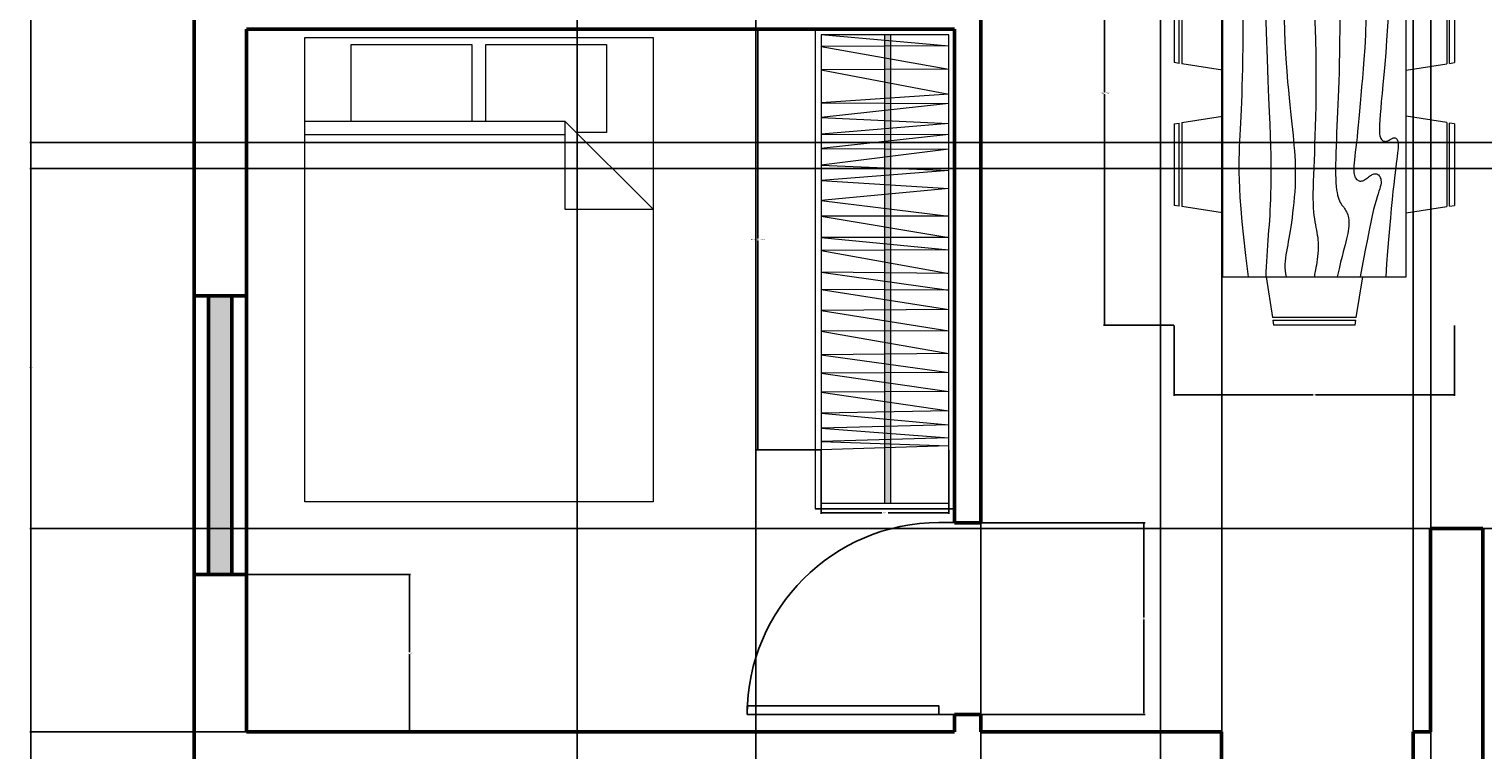
# Model space of a CAD drawing. Units: inches. Extents: x 1974 to 2406, y 1583 to 2170.
# Tile 3 of 6: x 1974 to 2224, y 1806 to 1930. Entities that reach past the tile are written whole.
import ezdxf

# ---------------------------------------------------------------- set-up
doc = ezdxf.new("R2010")
doc.units = ezdxf.units.IN
for name, color, linetype, lineweight in [('A-ANNO-DIMS', 2, 'Continuous', 18), ('A-FURN', 3, 'Continuous', 18), ('A-GLAZ', 4, 'Continuous', 25), ('door', 60, 'Continuous', 25), ('wall', 240, 'Continuous', 50)]:
    doc.layers.add(name, color=color, linetype=linetype, lineweight=lineweight)
doc.layers.add('A-FLOR-CASE', color=40, linetype='Continuous', lineweight=18, true_color=0xf8d731)
doc.layers.add('A-FLOR-CASE-PATT', color=40, linetype='Continuous', lineweight=13, true_color=0xf8d731)
doc.styles.get("Standard").update_dxf_attribs({"font": 'arial.ttf'})
doc.dimstyles.get("Standard").update_dxf_attribs({"dimtxt": 0.18, "dimasz": 0.18, "dimexe": 0.18, "dimexo": 0.0625, "dimgap": 0.09, "dimtad": 0, "dimtih": 1, "dimtoh": 1, "dimdec": 4, "dimzin": 0, "dimdsep": 46, "dimtxsty": 'Standard', "dimcen": 0.09, "dimadec": 0, "dimazin": 0, "dimtfac": 1, "dimtdec": 4, "dimtofl": 0, "dimtmove": 0, "dimatfit": 3, "dimfxl": 1, "dimtolj": 1, "dimtzin": 0, "dimarcsym": 0})

# ---------------------------------------------------------------- blocks, each defined once
blk = doc.blocks.new('*U2')
for p, q in [((0, 0), (0, -6)), ((40, 0), (40, -6))]:
    blk.add_line(p, q)
blk.add_lwpolyline([(0, 0), (0, 40), (1.75, 40), (1.75, 0)], close=True)
blk.add_arc((0, 0), 40, 0, 90)
blk = doc.blocks.new('b')
at = {"layer": 'wall'}
h = blk.add_hatch(color=256, dxfattribs=at)
h.dxf.hatch_style = 1
h.paths.add_polyline_path([(6.5, 0), (2.5, 0), (2.5, -48), (6.5, -48)])
for p, q in [((2.5, 0), (2.5, -48)), ((6.5, 0), (6.5, -48))]:
    blk.add_line(p, q, dxfattribs=at)
blk.add_lwpolyline([(0, -48), (9, -48), (9, 0), (0, 0)], close=True, dxfattribs=at)
blk = doc.blocks.new('Dining Set - 36 x 72 in.')
for p, q in [((-22.2343, 26.00059), (-23.4847, 17.99762)), ((-22.2304, 26), (-5.7608, 26)), ((-22, 27.5), (-22.1562, 26.50042)), ((-5.8416, 26.5), (-22.1534, 26.5)), ((-22, 27.5), (-6, 27.5)), ((-5.8437, 26.49966), (-6, 27.5)), ((-4.5152, 17.99762), (-5.7655, 25.99926)), ((5.7657, 26.00059), (4.5153, 17.99762)), ((5.7696, 26), (22.2392, 26)), ((6, 27.5), (5.8438, 26.50042)), ((22.1584, 26.5), (5.8466, 26.5)), ((6, 27.5), (22, 27.5)), ((22.1563, 26.49966), (22, 27.5)), ((23.4848, 17.99762), (22.2345, 25.99926)), ((36, 18), (-36, 18)), ((-36, 18), (-36, -18)), ((36, -18), (36, 18)), ((-44.0006, 8.23428), (-35.9976, 9.48474)), ((44.0006, 8.23428), (35.9976, 9.48474)), ((-45.5, 8), (-44.5004, 8.15617)), ((-45.5, 8), (-45.5, -8)), ((-44.5, -8.15843), (-44.5, 8.15338)), ((-44, 8.23041), (-44, -8.23915)), ((44, 8.23041), (44, -8.23915)), ((44.5, -8.15843), (44.5, 8.15338)), ((45.5, 8), (44.5005, 8.15617)), ((45.5, 8), (45.5, -8)), ((-44.4997, -8.15631), (-45.5, -8)), ((-35.9976, -9.48476), (-43.9993, -8.2345)), ((35.9976, -9.48476), (43.9993, -8.2345)), ((44.4997, -8.15631), (45.5, -8)), ((-36, -18), (36, -18)), ((-22.2343, -26.0006), (-23.4847, -17.99762)), ((-4.5152, -17.99762), (-5.7655, -25.99928)), ((5.7657, -26.0006), (4.5153, -17.99762)), ((23.4848, -17.99762), (22.2345, -25.99928)), ((-22.2304, -26), (-5.7608, -26)), ((-22, -27.5), (-22.1562, -26.50044)), ((-5.8416, -26.5), (-22.1534, -26.5)), ((-22, -27.5), (-6, -27.5)), ((-5.8437, -26.49967), (-6, -27.5)), ((5.7696, -26), (22.2392, -26)), ((6, -27.5), (5.8438, -26.50044)), ((22.1584, -26.5), (5.8466, -26.5)), ((6, -27.5), (22, -27.5)), ((22.1563, -26.49967), (22, -27.5))]:
    blk.add_line(p, q)
for points in [[(-36, 15), (-31.1772, 14.97754), (-26.8079, 14.91406), (-22.8538, 14.81543), (-19.276, 14.6875), (-16.0362, 14.53613), (-13.0957, 14.36718), (-10.4159, 14.18652), (-7.9583, 14), (-5.6904, 13.81315), (-3.6035, 13.63021), (-1.6954, 13.45508), (0.0365, 13.29166), (1.5945, 13.14388), (2.9811, 13.01562), (4.1988, 12.9108), (5.25, 12.83333), (6.1393, 12.78613), (6.8802, 12.76823), (7.4883, 12.77767), (7.9792, 12.8125), (8.3685, 12.87077), (8.6719, 12.95052), (8.9049, 13.0498), (9.0833, 13.16666), (9.2205, 13.29899), (9.3216, 13.44401), (9.3895, 13.59879), (9.4271, 13.76041), (9.4373, 13.92594), (9.4232, 14.09245), (9.3875, 14.257), (9.3333, 14.41666), (9.2638, 14.56917), (9.1836, 14.71484), (9.0975, 14.85465), (9.0104, 14.98958), (8.9272, 15.1206), (8.8529, 15.2487), (8.7922, 15.37483), (8.75, 15.5), (8.7305, 15.62467), (8.7344, 15.74739), (8.7617, 15.86621), (8.8125, 15.97916), (8.8867, 16.08431), (8.9844, 16.17968), (9.1055, 16.26334), (9.25, 16.33333), (9.4189, 16.38802), (9.6172, 16.42708), (9.8506, 16.45052), (10.125, 16.45833), (10.4463, 16.45052), (10.8203, 16.42708), (11.2529, 16.38802), (11.75, 16.33333), (12.3184, 16.26318), (12.9694, 16.17838), (13.7151, 16.07991), (14.5677, 15.96875), (15.5395, 15.84586), (16.6426, 15.71224), (17.8893, 15.56884), (19.2917, 15.41666), (20.859, 15.25667), (22.5879, 15.08984), (24.4721, 14.91715), (26.5052, 14.73958), (28.6809, 14.5581), (30.9929, 14.3737), (33.4347, 14.18733), (36, 14)], [(-36, 10), (-28.9766, 10.14274), (-23.1725, 10.20442), (-18.4241, 10.19775), (-14.5677, 10.13541), (-11.4399, 10.03011), (-8.877, 9.89453), (-6.7154, 9.74137), (-4.7917, 9.58333), (-2.9698, 9.43082), (-1.2246, 9.28515), (0.4415, 9.14534), (2.026, 9.01041), (3.5266, 8.87939), (4.9408, 8.7513), (6.266, 8.62516), (7.5, 8.5), (8.6411, 8.37549), (9.6914, 8.2539), (10.6538, 8.13818), (11.5312, 8.03125), (12.3267, 7.93603), (13.043, 7.85547), (13.6831, 7.79248), (14.25, 7.75), (14.7471, 7.7303), (15.1797, 7.73307), (15.5537, 7.75732), (15.875, 7.80208), (16.1494, 7.86637), (16.3828, 7.94922), (16.5811, 8.04964), (16.75, 8.16666), (16.8944, 8.29915), (17.0143, 8.44531), (17.1089, 8.60319), (17.1771, 8.77083), (17.218, 8.94629), (17.2305, 9.1276), (17.2137, 9.31282), (17.1667, 9.5), (17.0895, 9.6875), (16.987, 9.875), (16.8649, 10.0625), (16.7292, 10.25), (16.5856, 10.4375), (16.4401, 10.625), (16.2985, 10.8125), (16.1667, 11), (16.05, 11.18733), (15.9518, 11.3737), (15.8752, 11.5581), (15.8229, 11.73958), (15.798, 11.91715), (15.8034, 12.08984), (15.842, 12.25667), (15.9167, 12.41666), (16.0295, 12.56836), (16.1784, 12.70833), (16.3605, 12.83268), (16.5729, 12.9375), (16.8127, 13.01888), (17.0768, 13.07291), (17.3625, 13.0957), (17.6667, 13.08333), (17.9894, 13.03312), (18.3418, 12.94726), (18.7382, 12.82918), (19.1927, 12.68229), (19.7195, 12.51001), (20.3327, 12.31575), (21.0465, 12.10294), (21.875, 11.875), (22.8357, 11.63354), (23.959, 11.37304), (25.2786, 11.08618), (26.8282, 10.76562), (28.6414, 10.40405), (30.752, 9.99414), (33.1936, 9.52856), (36, 9)], [(-36, 5.5), (-30.7157, 5.3348), (-26.069, 5.20963), (-21.9946, 5.11767), (-18.4271, 5.05208), (-15.3009, 5.00602), (-12.5508, 4.97265), (-10.1112, 4.94515), (-7.9167, 4.91666), (-5.909, 4.88167), (-4.0586, 4.83984), (-2.3429, 4.79215), (-0.7396, 4.73958), (0.7739, 4.6831), (2.22, 4.6237), (3.6213, 4.56233), (5, 4.5), (6.373, 4.43782), (7.7344, 4.3776), (9.0723, 4.32129), (10.375, 4.27083), (11.6309, 4.22819), (12.8281, 4.19531), (13.9551, 4.17415), (15, 4.16666), (15.954, 4.17448), (16.819, 4.19791), (17.6001, 4.23698), (18.3021, 4.29166), (18.9299, 4.36198), (19.4883, 4.44791), (19.9823, 4.54948), (20.4167, 4.66666), (20.7969, 4.79899), (21.1302, 4.94401), (21.4245, 5.09879), (21.6875, 5.26041), (21.9271, 5.42594), (22.1511, 5.59245), (22.3672, 5.757), (22.5834, 5.91666), (22.8065, 6.06868), (23.0404, 6.21093), (23.2879, 6.34147), (23.5521, 6.45833), (23.8358, 6.55957), (24.142, 6.64323), (24.4735, 6.70735), (24.8334, 6.75), (25.2235, 6.76969), (25.642, 6.76692), (26.0858, 6.74267), (26.5521, 6.69791), (27.0379, 6.63362), (27.5404, 6.55078), (28.0565, 6.45036), (28.5834, 6.33333), (29.1242, 6.19987), (29.7071, 6.04687), (30.3661, 5.87044), (31.1354, 5.66666), (32.0493, 5.43164), (33.142, 5.16146), (34.4475, 4.85221), (36, 4.5)], [(-36, -1), (-30.7915, -0.6591), (-26.0195, -0.38216), (-21.6519, -0.16284), (-17.6563, 0.00521), (-14.0005, 0.12833), (-10.6523, 0.21289), (-7.5796, 0.26522), (-4.75, 0.29166), (-2.134, 0.29793), (0.2878, 0.28711), (2.5317, 0.26163), (4.6146, 0.22396), (6.5529, 0.17651), (8.3633, 0.12174), (10.0623, 0.06209), (11.6667, 0), (13.1899, -0.06201), (14.6341, -0.1211), (15.9982, -0.17432), (17.2813, -0.21875), (18.4823, -0.25147), (19.6003, -0.26953), (20.6343, -0.27002), (21.5834, -0.25), (22.4481, -0.20768), (23.2357, -0.14584), (23.9549, -0.06836), (24.6146, 0.02083), (25.2235, 0.11784), (25.7904, 0.21875), (26.3241, 0.31966), (26.8334, 0.41666), (27.3265, 0.50618), (27.8099, 0.58593), (28.2894, 0.65397), (28.7709, 0.70833), (29.2601, 0.74707), (29.763, 0.76823), (30.2855, 0.76985), (30.8334, 0.75), (31.4088, 0.70784), (31.9994, 0.64713), (32.589, 0.57275), (33.1615, 0.48958), (33.7008, 0.4025), (34.1908, 0.3164), (34.6153, 0.23616), (34.9584, 0.16666), (35.2099, 0.11165), (35.3848, 0.07031), (35.504, 0.04069), (35.5886, 0.02083), (35.6594, 0.00879), (35.7377, 0.0026), (35.8442, 0.00032), (36, 0)], [(-36, -6.5), (-27.1843, -6.31267), (-20.084, -6.1263), (-14.469, -5.9419), (-10.1094, -5.76042), (-6.7752, -5.58285), (-4.2363, -5.41016), (-2.2629, -5.24333), (-0.625, -5.08334), (0.8708, -4.93099), (2.2715, -4.78646), (3.5872, -4.64974), (4.8281, -4.52084), (6.0046, -4.39974), (7.127, -4.28646), (8.2053, -4.18099), (9.25, -4.08334), (10.2705, -3.99382), (11.2734, -3.91407), (12.2647, -3.84603), (13.25, -3.79167), (14.2354, -3.75293), (15.2266, -3.73177), (16.2295, -3.73015), (17.25, -3.75), (18.2912, -3.79248), (19.3451, -3.85547), (20.4009, -3.93604), (21.4479, -4.03125), (22.4754, -4.13819), (23.4727, -4.25391), (24.4289, -4.37549), (25.3334, -4.5), (26.1785, -4.62492), (26.9694, -4.74935), (27.7145, -4.87281), (28.4219, -4.99479), (29.1, -5.11483), (29.7572, -5.23242), (30.4016, -5.34709), (31.0417, -5.45834), (31.6837, -5.56437), (32.3262, -5.65821), (32.9658, -5.73153), (33.599, -5.77604), (34.2224, -5.78345), (34.8327, -5.74545), (35.4264, -5.65373), (36, -5.5)], [(-36, -10), (-26.4022, -9.81299), (-18.4675, -9.62891), (-11.9839, -9.45069), (-6.7396, -9.28125), (-2.5226, -9.12354), (0.8789, -8.98047), (3.6769, -8.85498), (6.0833, -8.75), (8.2767, -8.66765), (10.3021, -8.60677), (12.1712, -8.56543), (13.8958, -8.54167), (15.4876, -8.53353), (16.9583, -8.53907), (18.3197, -8.55632), (19.5834, -8.58334), (20.7616, -8.61841), (21.8685, -8.66081), (22.9188, -8.71004), (23.9271, -8.76563), (24.9081, -8.82707), (25.8763, -8.89388), (26.8465, -8.96558), (27.8334, -9.04167), (28.8474, -9.12118), (29.8828, -9.20117), (30.93, -9.27824), (31.9792, -9.34896), (33.0205, -9.40991), (34.0443, -9.45768), (35.0407, -9.48885), (36, -9.5)], [(-36, -14.5), (-30.0881, -14.33513), (-25.0332, -14.21224), (-20.7312, -14.12647), (-17.0781, -14.07292), (-13.97, -14.04671), (-11.3027, -14.04297), (-8.9724, -14.05681), (-6.875, -14.08334), (-4.9224, -14.11833), (-3.0905, -14.16016), (-1.3709, -14.20785), (0.2448, -14.26042), (1.7647, -14.3169), (3.1973, -14.3763), (4.5507, -14.43767), (5.8333, -14.5), (7.0554, -14.5621), (8.235, -14.62175), (9.3922, -14.67652), (10.5469, -14.72396), (11.7192, -14.76164), (12.929, -14.78711), (14.1965, -14.79794), (15.5417, -14.79167), (16.9933, -14.76424), (18.6152, -14.70508), (20.4804, -14.60197), (22.6615, -14.44271), (25.2312, -14.21509), (28.2624, -13.9069), (31.8277, -13.50594), (36, -13)]]:
    blk.add_lwpolyline(points)
blk = doc.blocks.new('Bed - Queen')
for p, q in [((0, -80.00003), (0, 0)), ((0, 0), (59.99999, 0)), ((59.99999, 0), (59.99999, -80.00003)), ((7.99999, -1.2), (28.79998, -1.2)), ((7.99999, -14.4), (7.99999, -1.2)), ((28.79998, -1.2), (28.79998, -14.4)), ((31.19999, -1.2), (51.99999, -1.2)), ((31.19999, -14.4), (31.19999, -1.2)), ((51.99999, -1.2), (51.99999, -16.4)), ((0, -14.4), (44.8, -14.4)), ((59.99999, -29.6), (44.8, -14.4)), ((44.8, -14.4), (44.8, -29.6)), ((44.8, -16.8), (0, -16.8)), ((51.99999, -16.4), (46.79936, -16.4)), ((44.8, -29.6), (59.99999, -29.6)), ((59.99999, -80.00003), (0, -80.00003))]:
    blk.add_line(p, q)
blk = doc.blocks.new('CLOSET-HANGER-RUN')
for p, q in [((0, 0), (0, 22)), ((0.94, 0), (2.86, 22)), ((2.86, 22), (2.99, 0)), ((2.99, 0), (6.93, 22)), ((6.93, 22), (6.99, 0)), ((6.99, 0), (11.19, 22)), ((11.19, 22), (12.71, 0)), ((12.71, 0), (12.83, 22)), ((12.83, 22), (15.2, 0)), ((15.2, 0), (16.24, 22)), ((16.24, 22), (18.1, 0)), ((18.1, 0), (18.16, 22)), ((18.16, 22), (20.55, 0)), ((20.55, 0), (20.68, 22)), ((20.68, 22), (23.44, 0)), ((23.44, 0), (24.36, 22)), ((24.36, 22), (26.08, 0)), ((26.08, 0), (27.44, 22)), ((27.44, 22), (29.52, 0)), ((29.52, 0), (32.2, 22)), ((32.2, 22), (32.2, 0)), ((32.2, 0), (35.87, 22)), ((35.87, 22), (35.87, 0)), ((35.87, 0), (38.02, 22)), ((38.02, 22), (38.12, 0)), ((38.12, 0), (42.07, 22)), ((42.07, 22), (41.87, 0)), ((41.87, 0), (44.93, 22)), ((44.93, 22), (44.83, 0)), ((44.83, 0), (48.29, 22)), ((48.29, 22), (48.48, 0)), ((48.48, 0), (51.94, 22)), ((51.94, 22), (52.04, 0)), ((52.04, 0), (55.89, 22)), ((55.89, 22), (56.08, 0)), ((56.08, 0), (59.14, 22)), ((59.14, 22), (59.24, 0)), ((59.24, 0), (62.4, 22)), ((62.4, 22), (62.5, 0)), ((62.5, 0), (65.76, 22)), ((65.76, 22), (66.15, 0)), ((66.15, 0), (68.13, 22)), ((68.13, 22), (68.72, 0)), ((68.72, 0), (70.4, 22)), ((70.4, 22), (70.99, 0)), ((70.99, 0), (71.78, 22)), ((71.78, 22), (72.44, 0))]:
    blk.add_line(p, q)
blk = doc.blocks.new('*D30')
at = {"layer": 'A-ANNO-DIMS', "color": 0, "lineweight": -2, "transparency": 16777216}
for p, q in [((2110.1, 1929.99), (2099.11, 1929.99)), ((2099.29, 1929.81), (2099.29, 1893.95)), ((2099.29, 1857.73), (2099.29, 1893.59)), ((2110.1, 1857.55), (2099.11, 1857.55))]:
    blk.add_line(p, q, dxfattribs=at)
at = {"layer": 'A-ANNO-DIMS', "color": 0, "transparency": 16777216}
for points in [[(2099.26, 1929.81), (2099.32, 1929.81), (2099.29, 1929.99)], [(2099.26, 1857.73), (2099.32, 1857.73), (2099.29, 1857.55)]]:
    blk.add_solid(points, dxfattribs=at)
at = {"layer": 'Defpoints', "color": 0, "transparency": 16777216}
for p in [(2110.16, 1929.99), (2099.29, 1857.55), (2110.16, 1857.55)]:
    blk.add_point(p, dxfattribs=at)
at = {"layer": 'A-ANNO-DIMS', "color": 0, "transparency": 16777216, "insert": (2099.29, 1893.77), "char_height": 0.18, "attachment_point": 5}
blk.add_mtext('\\A1;HANGER RUN 72 TYP.', dxfattribs=at)
blk = doc.blocks.new('*D31')
at = {"layer": 'A-ANNO-DIMS', "color": 0, "lineweight": -2, "transparency": 16777216}
for p, q in [((2110.16, 1857.49), (2110.16, 1846.5)), ((2132.16, 1857.49), (2132.16, 1846.5)), ((2110.34, 1846.68), (2120.63, 1846.68)), ((2131.98, 1846.68), (2121.69, 1846.68))]:
    blk.add_line(p, q, dxfattribs=at)
at = {"layer": 'A-ANNO-DIMS', "color": 0, "transparency": 16777216}
for points in [[(2110.34, 1846.71), (2110.34, 1846.65), (2110.16, 1846.68)], [(2131.98, 1846.71), (2131.98, 1846.65), (2132.16, 1846.68)]]:
    blk.add_solid(points, dxfattribs=at)
at = {"layer": 'Defpoints', "color": 0, "transparency": 16777216}
for p in [(2110.16, 1857.55), (2132.16, 1857.55), (2132.16, 1846.68)]:
    blk.add_point(p, dxfattribs=at)
at = {"layer": 'A-ANNO-DIMS', "color": 0, "transparency": 16777216, "insert": (2121.16, 1846.68), "char_height": 0.18, "attachment_point": 5}
blk.add_mtext('\\A1;22 TYP.', dxfattribs=at)
blk = doc.blocks.new('*D42')
at = {"layer": 'A-ANNO-DIMS', "color": 0, "lineweight": -2, "transparency": 16777216}
for p, q in [((2170.92, 1958.88), (2158.82, 1958.88)), ((2159, 1958.7), (2159, 1919.13)), ((2159, 1879.18), (2159, 1918.76)), ((2170.92, 1879), (2158.82, 1879))]:
    blk.add_line(p, q, dxfattribs=at)
at = {"layer": 'A-ANNO-DIMS', "color": 0, "transparency": 16777216}
for points in [[(2158.97, 1958.7), (2159.03, 1958.7), (2159, 1958.88)], [(2158.97, 1879.18), (2159.03, 1879.18), (2159, 1879)]]:
    blk.add_solid(points, dxfattribs=at)
at = {"layer": 'Defpoints', "color": 0, "transparency": 16777216}
for p in [(2170.98, 1958.88), (2159, 1879), (2170.98, 1879)]:
    blk.add_point(p, dxfattribs=at)
at = {"layer": 'A-ANNO-DIMS', "color": 0, "transparency": 16777216, "insert": (2159, 1918.94), "char_height": 0.18, "attachment_point": 5}
blk.add_mtext('\\A1;DINING SET 80', dxfattribs=at)
blk = doc.blocks.new('*D43')
at = {"layer": 'A-ANNO-DIMS', "color": 0, "lineweight": -2, "transparency": 16777216}
for p, q in [((2170.98, 1878.94), (2170.98, 1866.84)), ((2219.26, 1878.94), (2219.26, 1866.84)), ((2171.16, 1867.02), (2194.9, 1867.02)), ((2219.08, 1867.02), (2195.34, 1867.02))]:
    blk.add_line(p, q, dxfattribs=at)
at = {"layer": 'A-ANNO-DIMS', "color": 0, "transparency": 16777216}
for points in [[(2171.16, 1867.05), (2171.16, 1866.99), (2170.98, 1867.02)], [(2219.08, 1867.05), (2219.08, 1866.99), (2219.26, 1867.02)]]:
    blk.add_solid(points, dxfattribs=at)
at = {"layer": 'Defpoints', "color": 0, "transparency": 16777216}
for p in [(2170.98, 1879), (2219.26, 1879), (2219.26, 1867.02)]:
    blk.add_point(p, dxfattribs=at)
at = {"layer": 'A-ANNO-DIMS', "color": 0, "transparency": 16777216, "insert": (2195.12, 1867.02), "char_height": 0.18, "attachment_point": 5}
blk.add_mtext('\\A1;48', dxfattribs=at)
blk = doc.blocks.new('*D56')
at = {"layer": 'A-ANNO-DIMS', "color": 0, "lineweight": -2, "transparency": 16777216}
for p, q in [((2011.1, 1934.49), (1973.86, 1934.49)), ((1974.04, 1934.31), (1974.04, 1871.92)), ((1974.04, 1809.17), (1974.04, 1871.56)), ((2011.1, 1808.99), (1973.86, 1808.99))]:
    blk.add_line(p, q, dxfattribs=at)
at = {"layer": 'A-ANNO-DIMS', "color": 0, "transparency": 16777216}
for points in [[(1974.01, 1934.31), (1974.07, 1934.31), (1974.04, 1934.49)], [(1974.01, 1809.17), (1974.07, 1809.17), (1974.04, 1808.99)]]:
    blk.add_solid(points, dxfattribs=at)
at = {"layer": 'Defpoints', "color": 0, "transparency": 16777216}
for p in [(2011.16, 1934.49), (1974.04, 1808.99), (2011.16, 1808.99)]:
    blk.add_point(p, dxfattribs=at)
at = {"layer": 'A-ANNO-DIMS', "color": 0, "transparency": 16777216, "insert": (1974.04, 1871.74), "char_height": 0.18, "attachment_point": 5}
blk.add_mtext('\\A1;125.5', dxfattribs=at)
blk = doc.blocks.new('*D57')
at = {"layer": 'A-ANNO-DIMS', "color": 0, "lineweight": -2, "transparency": 16777216}
for p, q in [((2011.1, 1808.99), (1973.86, 1808.99)), ((1974.04, 1808.81), (1974.04, 1752.17)), ((1974.04, 1695.17), (1974.04, 1751.81)), ((2002.1, 1694.99), (1973.86, 1694.99))]:
    blk.add_line(p, q, dxfattribs=at)
at = {"layer": 'A-ANNO-DIMS', "color": 0, "transparency": 16777216}
for points in [[(1974.01, 1808.81), (1974.07, 1808.81), (1974.04, 1808.99)], [(1974.01, 1695.17), (1974.07, 1695.17), (1974.04, 1694.99)]]:
    blk.add_solid(points, dxfattribs=at)
at = {"layer": 'Defpoints', "color": 0, "transparency": 16777216}
for p in [(2011.16, 1808.99), (1974.04, 1694.99), (2002.16, 1694.99)]:
    blk.add_point(p, dxfattribs=at)
at = {"layer": 'A-ANNO-DIMS', "color": 0, "transparency": 16777216, "insert": (1974.04, 1751.99), "char_height": 0.18, "attachment_point": 5}
blk.add_mtext('\\A1;114', dxfattribs=at)
blk = doc.blocks.new('*D70')
at = {"layer": 'A-ANNO-DIMS', "color": 0, "lineweight": -2, "transparency": 16777216}
for p, q in [((2137.72, 1844.99), (2165.96, 1844.99)), ((2165.78, 1844.81), (2165.78, 1828.67)), ((2165.78, 1812.17), (2165.78, 1828.31)), ((2137.72, 1811.99), (2165.96, 1811.99))]:
    blk.add_line(p, q, dxfattribs=at)
at = {"layer": 'A-ANNO-DIMS', "color": 0, "transparency": 16777216}
for points in [[(2165.75, 1844.81), (2165.81, 1844.81), (2165.78, 1844.99)], [(2165.75, 1812.17), (2165.81, 1812.17), (2165.78, 1811.99)]]:
    blk.add_solid(points, dxfattribs=at)
at = {"layer": 'Defpoints', "color": 0, "transparency": 16777216}
for p in [(2137.66, 1844.99), (2137.66, 1811.99), (2165.78, 1811.99)]:
    blk.add_point(p, dxfattribs=at)
at = {"layer": 'A-ANNO-DIMS', "color": 0, "transparency": 16777216, "insert": (2165.78, 1828.49), "char_height": 0.18, "attachment_point": 5}
blk.add_mtext('\\A1;33', dxfattribs=at)
blk = doc.blocks.new('*D71')
at = {"layer": 'A-ANNO-DIMS', "color": 0, "lineweight": -2, "transparency": 16777216}
for p, q in [((2011.22, 1836.08), (2039.46, 1836.08)), ((2039.28, 1835.9), (2039.28, 1822.72)), ((2039.28, 1809.17), (2039.28, 1822.36)), ((2011.22, 1808.99), (2039.46, 1808.99))]:
    blk.add_line(p, q, dxfattribs=at)
at = {"layer": 'A-ANNO-DIMS', "color": 0, "transparency": 16777216}
for points in [[(2039.25, 1835.9), (2039.31, 1835.9), (2039.28, 1836.08)], [(2039.25, 1809.17), (2039.31, 1809.17), (2039.28, 1808.99)]]:
    blk.add_solid(points, dxfattribs=at)
at = {"layer": 'Defpoints', "color": 0, "transparency": 16777216}
for p in [(2011.16, 1836.08), (2011.16, 1808.99), (2039.28, 1808.99)]:
    blk.add_point(p, dxfattribs=at)
at = {"layer": 'A-ANNO-DIMS', "color": 0, "transparency": 16777216, "insert": (2039.28, 1822.54), "char_height": 0.18, "attachment_point": 5}
blk.add_mtext('\\A1;27.09', dxfattribs=at)
blk = doc.blocks.new('*D73')
at = {"layer": 'A-ANNO-DIMS', "color": 0, "lineweight": -2, "transparency": 16777216}
for p, q in [((2258.6, 1972.49), (1973.86, 1972.49)), ((1974.04, 1972.31), (1974.04, 1941.67)), ((1974.04, 1910.67), (1974.04, 1941.31)), ((2254.1, 1910.49), (1973.86, 1910.49))]:
    blk.add_line(p, q, dxfattribs=at)
at = {"layer": 'A-ANNO-DIMS', "color": 0, "transparency": 16777216}
for points in [[(1974.01, 1972.31), (1974.07, 1972.31), (1974.04, 1972.49)], [(1974.01, 1910.67), (1974.07, 1910.67), (1974.04, 1910.49)]]:
    blk.add_solid(points, dxfattribs=at)
at = {"layer": 'Defpoints', "color": 0, "transparency": 16777216}
for p in [(2258.66, 1972.49), (1974.04, 1910.49), (2254.16, 1910.49)]:
    blk.add_point(p, dxfattribs=at)
at = {"layer": 'A-ANNO-DIMS', "color": 0, "transparency": 16777216, "insert": (1974.04, 1941.49), "char_height": 0.18, "attachment_point": 5}
blk.add_mtext('\\A1;62', dxfattribs=at)
blk = doc.blocks.new('*D75')
at = {"layer": 'A-ANNO-DIMS', "color": 0, "lineweight": -2, "transparency": 16777216}
for p, q in [((2258.6, 1905.99), (1973.86, 1905.99)), ((1974.04, 1905.81), (1974.04, 1875.17)), ((1974.04, 1844.17), (1974.04, 1874.81)), ((2258.6, 1843.99), (1973.86, 1843.99))]:
    blk.add_line(p, q, dxfattribs=at)
at = {"layer": 'A-ANNO-DIMS', "color": 0, "transparency": 16777216}
for points in [[(1974.01, 1905.81), (1974.07, 1905.81), (1974.04, 1905.99)], [(1974.01, 1844.17), (1974.07, 1844.17), (1974.04, 1843.99)]]:
    blk.add_solid(points, dxfattribs=at)
at = {"layer": 'Defpoints', "color": 0, "transparency": 16777216}
for p in [(2258.66, 1905.99), (1974.04, 1843.99), (2258.66, 1843.99)]:
    blk.add_point(p, dxfattribs=at)
at = {"layer": 'A-ANNO-DIMS', "color": 0, "transparency": 16777216, "insert": (1974.04, 1874.99), "char_height": 0.18, "attachment_point": 5}
blk.add_mtext('\\A1;62', dxfattribs=at)
blk = doc.blocks.new('*D89')
at = {"layer": 'A-ANNO-DIMS', "color": 0, "lineweight": -2, "transparency": 16777216}
for p, q in [((2179.16, 1809.05), (2179.16, 2170.29)), ((2179.34, 2170.11), (2195.44, 2170.11)), ((2211.98, 2170.11), (2195.88, 2170.11)), ((2212.16, 1809.05), (2212.16, 2170.29))]:
    blk.add_line(p, q, dxfattribs=at)
at = {"layer": 'A-ANNO-DIMS', "color": 0, "transparency": 16777216}
for points in [[(2179.34, 2170.14), (2179.34, 2170.08), (2179.16, 2170.11)], [(2211.98, 2170.14), (2211.98, 2170.08), (2212.16, 2170.11)]]:
    blk.add_solid(points, dxfattribs=at)
at = {"layer": 'Defpoints', "color": 0, "transparency": 16777216}
for p in [(2212.16, 2170.11), (2179.16, 1808.99), (2212.16, 1808.99)]:
    blk.add_point(p, dxfattribs=at)
at = {"layer": 'A-ANNO-DIMS', "color": 0, "transparency": 16777216, "insert": (2195.66, 2170.11), "char_height": 0.18, "attachment_point": 5}
blk.add_mtext('\\A1;33', dxfattribs=at)
blk = doc.blocks.new('*D92')
at = {"layer": 'A-ANNO-DIMS', "color": 0, "lineweight": -2, "transparency": 16777216}
for p, q in [((2168.64, 1725.52), (2168.64, 2170.29)), ((2168.82, 2170.11), (2191.5, 2170.11)), ((2214.98, 2170.11), (2192.3, 2170.11)), ((2215.16, 1728.05), (2215.16, 2170.29))]:
    blk.add_line(p, q, dxfattribs=at)
at = {"layer": 'A-ANNO-DIMS', "color": 0, "transparency": 16777216}
for points in [[(2168.82, 2170.14), (2168.82, 2170.08), (2168.64, 2170.11)], [(2214.98, 2170.14), (2214.98, 2170.08), (2215.16, 2170.11)]]:
    blk.add_solid(points, dxfattribs=at)
at = {"layer": 'Defpoints', "color": 0, "transparency": 16777216}
for p in [(2215.16, 2170.11), (2215.16, 1727.99), (2168.64, 1725.46)]:
    blk.add_point(p, dxfattribs=at)
at = {"layer": 'A-ANNO-DIMS', "color": 0, "transparency": 16777216, "insert": (2191.9, 2170.11), "char_height": 0.18, "attachment_point": 5}
blk.add_mtext('\\A1;46.52', dxfattribs=at)
blk = doc.blocks.new('*D93')
at = {"layer": 'A-ANNO-DIMS', "color": 0, "lineweight": -2, "transparency": 16777216}
for p, q in [((2068.16, 1728.05), (2068.16, 2170.29)), ((2068.34, 2170.11), (2083.07, 2170.11)), ((2098.72, 2170.11), (2083.99, 2170.11)), ((2098.9, 1721.56), (2098.9, 2170.29))]:
    blk.add_line(p, q, dxfattribs=at)
at = {"layer": 'A-ANNO-DIMS', "color": 0, "transparency": 16777216}
for points in [[(2068.34, 2170.14), (2068.34, 2170.08), (2068.16, 2170.11)], [(2098.72, 2170.14), (2098.72, 2170.08), (2098.9, 2170.11)]]:
    blk.add_solid(points, dxfattribs=at)
at = {"layer": 'Defpoints', "color": 0, "transparency": 16777216}
for p in [(2098.9, 2170.11), (2068.16, 1727.99), (2098.9, 1721.49)]:
    blk.add_point(p, dxfattribs=at)
at = {"layer": 'A-ANNO-DIMS', "color": 0, "transparency": 16777216, "insert": (2083.53, 2170.11), "char_height": 0.18, "attachment_point": 5}
blk.add_mtext('\\A1;30.746', dxfattribs=at)
blk = doc.blocks.new('*D94')
at = {"layer": 'A-ANNO-DIMS', "color": 0, "lineweight": -2, "transparency": 16777216}
for p, q in [((2068.16, 1800.05), (2068.16, 2170.29)), ((2068.34, 2170.11), (2102.58, 2170.11)), ((2137.48, 2170.11), (2103.23, 2170.11)), ((2137.66, 1800.05), (2137.66, 2170.29))]:
    blk.add_line(p, q, dxfattribs=at)
at = {"layer": 'A-ANNO-DIMS', "color": 0, "transparency": 16777216}
for points in [[(2068.34, 2170.14), (2068.34, 2170.08), (2068.16, 2170.11)], [(2137.48, 2170.14), (2137.48, 2170.08), (2137.66, 2170.11)]]:
    blk.add_solid(points, dxfattribs=at)
at = {"layer": 'Defpoints', "color": 0, "transparency": 16777216}
for p in [(2137.66, 2170.11), (2068.16, 1799.99), (2137.66, 1799.99)]:
    blk.add_point(p, dxfattribs=at)
at = {"layer": 'A-ANNO-DIMS', "color": 0, "transparency": 16777216, "insert": (2102.91, 2170.11), "char_height": 0.18, "attachment_point": 5}
blk.add_mtext('\\A1;69.5', dxfattribs=at)

msp = doc.modelspace()

# ---------------------------------------------------------------- hatches: boundary and pattern name
at = {"layer": 'A-FLOR-CASE-PATT'}
h = msp.add_hatch(color=256, dxfattribs=at)
h.dxf.hatch_style = 1
h.paths.add_polyline_path([(2122.1581, 1928.9921), (2121.1581, 1928.9921), (2121.1581, 1848.3602), (2122.1581, 1848.3602)])

# ---------------------------------------------------------------- linework, layer by layer
at = {"layer": 'A-FLOR-CASE'}
for p, q in [((2109.1581, 1929.9921), (2109.1581, 1847.3602)), ((2121.1581, 1848.3602), (2121.1581, 1928.9921)), ((2122.1581, 1848.3602), (2122.1581, 1928.9921)), ((2133.1581, 1847.3602), (2109.1581, 1847.3602))]:
    msp.add_line(p, q, dxfattribs=at)
for points in [[(2133.1581, 1929.9921), (2109.1581, 1929.9921), (2109.1581, 1847.3602), (2133.1581, 1847.3602)], [(2132.1581, 1928.9921), (2110.1581, 1928.9921), (2110.1581, 1848.3602), (2132.1581, 1848.3602)]]:
    msp.add_lwpolyline(points, close=True, dxfattribs=at)
at = {"layer": 'wall'}
for p, q in [((2002.1581, 2141.9921), (2002.1581, 1694.9921)), ((2137.6581, 1996.4921), (2137.6581, 1844.9921)), ((2011.1581, 1929.9921), (2133.1581, 1929.9921)), ((2011.1581, 1929.9921), (2011.1581, 1808.9921)), ((2133.1581, 1929.9921), (2133.1581, 1844.9921)), ((2137.6581, 1844.9921), (2133.1581, 1844.9921)), ((2215.1581, 1843.9921), (2224.1581, 1843.9921)), ((2215.1581, 1843.9921), (2215.1581, 1808.9921)), ((2224.1581, 1839.4921), (2224.1581, 1843.9921)), ((2224.1581, 1839.4921), (2224.1581, 1703.9921)), ((2137.6581, 1811.9921), (2133.1581, 1811.9921)), ((2133.1581, 1811.9921), (2133.1581, 1808.9921)), ((2137.6581, 1808.9921), (2137.6581, 1811.9921)), ((2137.6581, 1811.9921), (2137.6581, 1808.9921)), ((2011.1581, 1808.9921), (2133.1581, 1808.9921)), ((2137.6581, 1808.9921), (2179.1581, 1808.9921)), ((2179.1581, 1808.9921), (2179.1581, 1799.9921)), ((2215.1581, 1808.9921), (2212.1581, 1808.9921)), ((2212.1581, 1799.9921), (2212.1581, 1808.9921)), ((2212.1581, 1808.9921), (2215.1581, 1808.9921))]:
    msp.add_line(p, q, dxfattribs=at)

# ---------------------------------------------------------------- block references
at = {"layer": 'A-FLOR-CASE', "rotation": 270.0000000000053}
msp.add_blockref('CLOSET-HANGER-RUN', (2110.1579, 1929.9921), dxfattribs=at)
at = {"layer": 'A-FURN', "xscale": 0.8778001079660128, "yscale": 0.8778001079660128, "zscale": 0.8778001079660128, "rotation": 270}
msp.add_blockref('Dining Set - 36 x 72 in.', (2195.122, 1918.9446), dxfattribs=at)
at = {"layer": 'A-FURN'}
msp.add_blockref('Bed - Queen', (2021.2233, 1928.5592), dxfattribs=at)
at = {"layer": 'A-GLAZ'}
msp.add_blockref('b', (2002.1581, 1884.0832), dxfattribs=at)
at = {"layer": 'door', "xscale": 0.8252274917434117, "yscale": 0.8252274917434117, "zscale": 0.8252274917434117, "rotation": 90.00000000000003}
msp.add_blockref('*U2', (2130.4567, 1811.9921), dxfattribs=at)

# ---------------------------------------------------------------- dimensions: what is measured, and where the dimension line sits
at = {"layer": 'A-ANNO-DIMS'}
for base, p1, p2, override, picture, middle in [((2098.9039, 2170.1096), (2068.1581, 1727.9921), (2098.9039, 1721.4943), {"dimdec": 3, "dimlfac": 1, "dimrnd": 0, "dimzin": 0, "dimdsep": 46, "dimlunit": 2}, '*D93', (2083.531, 2170.1096)), ((2137.6581, 2170.1096), (2068.1581, 1799.9921), (2137.6581, 1799.9921), {"dimdec": 1, "dimlfac": 1, "dimrnd": 0, "dimzin": 0, "dimdsep": 46, "dimlunit": 2}, '*D94', (2102.9081, 2170.1096)), ((2215.1581, 2170.1096), (2168.6394, 1725.4624), (2215.1581, 1727.9921), {"dimdec": 2, "dimlfac": 1, "dimrnd": 0, "dimzin": 0, "dimdsep": 46, "dimlunit": 2}, '*D92', (2191.8987, 2170.1096)), ((2212.1581, 2170.1096), (2179.1581, 1808.9921), (2212.1581, 1808.9921), {"dimdec": 0, "dimlfac": 1, "dimrnd": 0, "dimzin": 0, "dimdsep": 46, "dimlunit": 2}, '*D89', (2195.6581, 2170.1096)), ((2219.2615, 1867.0227), (2170.9825, 1879.0047), (2219.2615, 1879.0047), {"dimdec": 0, "dimlfac": 1, "dimrnd": 0, "dimzin": 0, "dimdsep": 46, "dimlunit": 2}, '*D43', (2195.122, 1867.0227))]:
    dim = msp.add_linear_dim(base=base, p1=p1, p2=p2, dimstyle='Standard', override=override, dxfattribs=at)
    dim.commit()
    dim.dimension.update_dxf_attribs({"geometry": picture, "text_midpoint": middle})
for base, p1, p2, angle, override, picture, middle in [((1974.0406, 1910.4921), (2258.6581, 1972.4921), (2254.1581, 1910.4921), 90, {"dimdec": 0, "dimlfac": 1, "dimrnd": 0, "dimzin": 0, "dimdsep": 46, "dimlunit": 2}, '*D73', (1974.0406, 1941.4921)), ((1974.0406, 1808.9921), (2011.1581, 1934.4921), (2011.1581, 1808.9921), 90, {"dimdec": 1, "dimlfac": 1, "dimrnd": 0, "dimzin": 0, "dimdsep": 46, "dimlunit": 2}, '*D56', (1974.0406, 1871.7421)), ((1974.0406, 1843.9921), (2258.6581, 1905.9921), (2258.6581, 1843.9921), 90, {"dimdec": 0, "dimlfac": 1, "dimrnd": 0, "dimzin": 0, "dimdsep": 46, "dimlunit": 2}, '*D75', (1974.0406, 1874.9921)), ((2165.7756, 1811.9921), (2137.6581, 1844.9921), (2137.6581, 1811.9921), 270, {"dimdec": 0, "dimlfac": 1, "dimrnd": 0, "dimzin": 0, "dimdsep": 46, "dimlunit": 2}, '*D70', (2165.7756, 1828.4921)), ((2039.2756, 1808.9921), (2011.1581, 1836.0832), (2011.1581, 1808.9921), 270, {"dimdec": 2, "dimlfac": 1, "dimrnd": 0, "dimzin": 0, "dimdsep": 46, "dimlunit": 2}, '*D71', (2039.2756, 1822.5377)), ((1974.0406, 1694.9921), (2011.1581, 1808.9921), (2002.1581, 1694.9921), 90, {"dimdec": 0, "dimlfac": 1, "dimrnd": 0, "dimzin": 0, "dimdsep": 46, "dimlunit": 2}, '*D57', (1974.0406, 1751.9921))]:
    dim = msp.add_linear_dim(base=base, p1=p1, p2=p2, angle=angle, dimstyle='Standard', override=override, dxfattribs=at)
    dim.commit()
    dim.dimension.update_dxf_attribs({"geometry": picture, "text_midpoint": middle})
for base, p1, p2, angle, text, picture, middle in [((2159.0005, 1879.0047), (2170.9825, 1958.8845), (2170.9825, 1879.0047), 270, 'DINING SET <>', '*D42', (2159.0005, 1918.9446)), ((2099.2916, 1857.5488), (2110.1581, 1929.9921), (2110.1581, 1857.5488), 270, 'HANGER RUN <> TYP.', '*D30', (2099.2916, 1893.7705)), ((2132.1581, 1846.6823), (2110.1581, 1857.5488), (2132.1581, 1857.5488), 0, '<> TYP.', '*D31', (2121.1581, 1846.6823))]:
    dim = msp.add_linear_dim(base=base, p1=p1, p2=p2, angle=angle, text=text, dimstyle='Standard', override={"dimdec": 0, "dimlfac": 1, "dimrnd": 0, "dimzin": 0, "dimdsep": 46, "dimlunit": 2}, dxfattribs=at)
    dim.commit()
    dim.dimension.update_dxf_attribs({"geometry": picture, "text_midpoint": middle})

doc.saveas('drawing.dxf')
